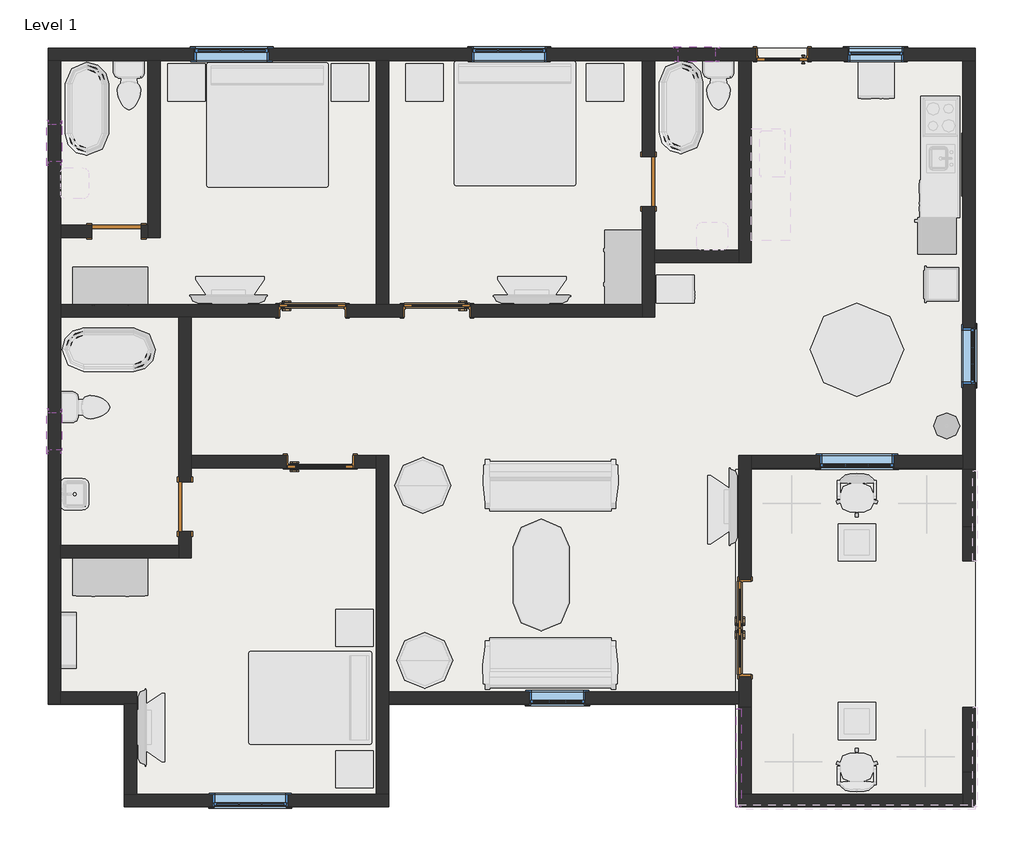
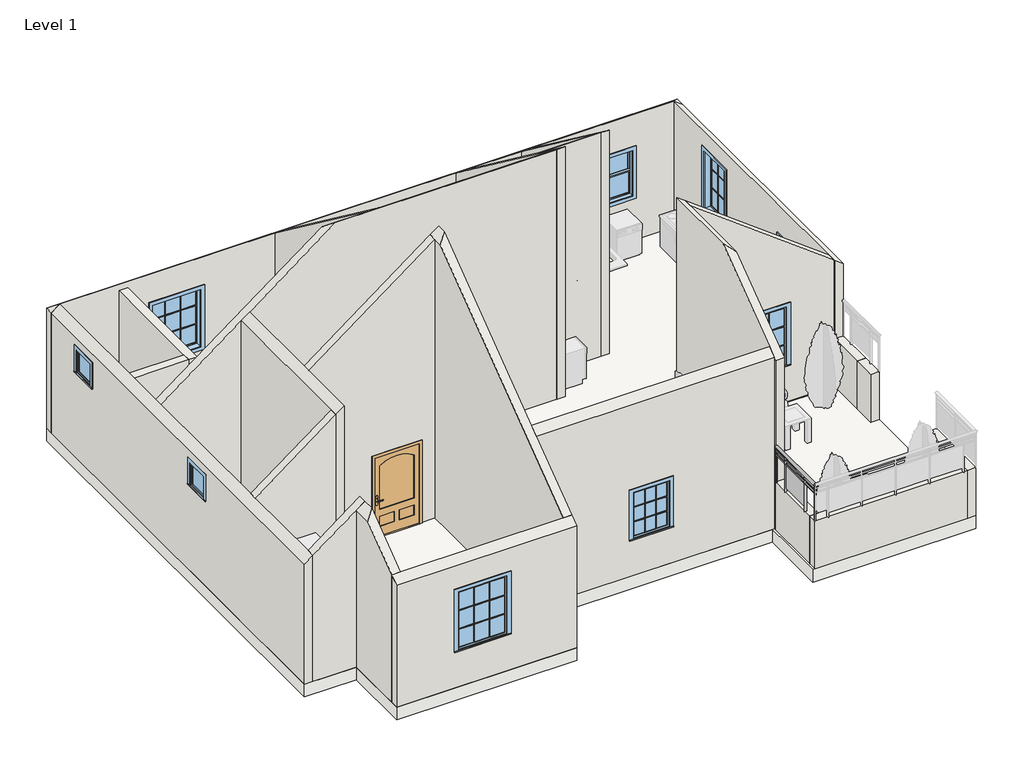
# One storey, part 1 of 2: 26 walls, 11 windows, 8 doors, 2 slabs, 1 railing.
"""IFC4 building model written with IfcOpenShell, lengths in millimetres."""

from ifc_helpers import new_model, si_unit, point, frame, origin, origin_with_axes, place, context, project, spatial, polyline, ellipse_curve, trimmed, outline, extrude, faceted_brep, transform, mapped, element, save
from ifc_brep_helpers import plane_surface, extruded_surface, advanced_brep
from components import door_fa6f8c62, door_3b8e8068, door_b03bd389, door_22967355, door_0d629d65, door_64d5ae29, window_29c06734, window_58e1470a, window_99fc0ff6, window_31198920, window_e41d21a6

model = new_model("IFC4")

# Units and contexts
model_context = context("Model", 3, world=origin())
ifc_project = project(units=[si_unit("LENGTHUNIT", "METRE", prefix="MILLI")], contexts=[model_context])

# Site, building, storey
site = spatial("IfcSite", under=ifc_project)
building = spatial("IfcBuilding", under=site)
storey = spatial("IfcBuildingStorey", under=building, Name="Level 1", Elevation=0.0)

# Doors
placement = place(None, origin())
door_shape = door_fa6f8c62(model_context)
element("IfcDoor", 1, ObjectType="42\" x 80\"", at=placement, inside=storey, context=model_context, shape_type="MappedRepresentation", body=[
    mapped(door_shape, transform((-8993.195199, 2667.0826725, 0.0), x_axis=(-1.0, 0.0, 0.0), y_axis=(0.0, -1.0, 0.0), z_axis=(0.0, 0.0, 1.0))),
])
door_2_shape = door_3b8e8068(model_context)
element("IfcDoor", 2, ObjectType="42\" x 80\"", at=placement, inside=storey, context=model_context, shape_type="MappedRepresentation", body=[
    mapped(door_2_shape, transform((-6961.195199, 2667.0826725, 0.0), x_axis=(1.0, 0.0, 0.0), y_axis=(0.0, 1.0, 0.0), z_axis=(0.0, 0.0, 1.0))),
])
element("IfcDoor", 3, ObjectType="42\" x 80\"", at=placement, inside=storey, context=model_context, shape_type="MappedRepresentation", body=[
    mapped(door_2_shape, transform((-8866.195199, 196.9326725, 0.0), x_axis=(-1.0, 0.0, 0.0), y_axis=(0.0, -1.0, 0.0), z_axis=(0.0, 0.0, 1.0))),
])
door_3_shape = door_b03bd389(model_context)
element("IfcDoor", 4, ObjectType="Door-Exterior-Double-Full Glass-Wood_Clad : 60\" x 80\"", at=placement, inside=storey, context=model_context, shape_type="MappedRepresentation", body=[
    mapped(door_3_shape, transform((-1935.170199, -2517.6923275, 0.0), x_axis=(0.0, 1.0, 0.0), y_axis=(-1.0, 0.0, 0.0), z_axis=(0.0, 0.0, 1.0))),
])
door_4_shape = door_22967355(model_context)
element("IfcDoor", 5, ObjectType="Door-Interior-Single-Full Glass-Wood : 32\" x 80\"", at=placement, inside=storey, context=model_context, shape_type="MappedRepresentation", body=[
    mapped(door_4_shape, transform((-1322.395199, 6851.7326725, 0.0), x_axis=(-1.0, 0.0, 0.0), y_axis=(0.0, -1.0, 0.0), z_axis=(0.0, 0.0, 1.0))),
])
door_5_shape = door_0d629d65(model_context)
element("IfcDoor", 6, ObjectType="Single-Flush : 32\" x 84\"", at=placement, inside=storey, context=model_context, shape_type="MappedRepresentation", body=[
    mapped(door_5_shape, transform((-11075.995199, -536.4923275, 0.0), x_axis=(0.0, -1.0, 0.0), y_axis=(1.0, 0.0, 0.0), z_axis=(0.0, 0.0, 1.0))),
])
door_6_shape = door_64d5ae29(model_context)
element("IfcDoor", 7, ObjectType="Single-Flush : 32\" x 84\"", at=placement, inside=storey, context=model_context, shape_type="MappedRepresentation", body=[
    mapped(door_6_shape, transform((-3506.795199, 4772.1076725, 0.0), x_axis=(0.0, -1.0, 0.0), y_axis=(1.0, 0.0, 0.0), z_axis=(0.0, 0.0, 1.0))),
])
element("IfcDoor", 8, ObjectType="Single-Flush : 32\" x 84\"", at=placement, inside=storey, context=model_context, shape_type="MappedRepresentation", body=[
    mapped(door_6_shape, transform((-12193.595199, 3959.3076725, 0.0), x_axis=(1.0, 0.0, 0.0), y_axis=(0.0, 1.0, 0.0), z_axis=(0.0, 0.0, 1.0))),
])

# Railing
element("IfcRailing", 9, ObjectType="Glass Panel - Bottom Fill", at=placement, inside=storey, context=model_context, shape_type="SolidModel", body=[
    advanced_brep(
    [(-1995.495199, -3838.4923275, 2133.6), (-2071.695199, -3838.4923275, 2133.6), (-1995.495199, -5438.6923275, 2133.6), (-2071.695199, -5438.6923275, 2133.6)],
    [
        (0, 1, ellipse_curve(frame((-2033.595199, -3838.4923275, 2133.6), z_axis=(0.0, 1.0, 0.0), x_axis=(-1.0, 0.0, 0.0)), 38.1, 28.575)),
        (1, 0, ellipse_curve(frame((-2033.595199, -3838.4923275, 2133.6), z_axis=(0.0, 1.0, 0.0), x_axis=(-1.0, 0.0, 0.0)), 38.1, 28.575)),
        (2, 3, ellipse_curve(frame((-2033.595199, -5438.6923275, 2133.6), z_axis=(0.0, -1.0, 0.0), x_axis=(-1.0, 0.0, 0.0)), 38.1, 28.575)),
        (3, 2, ellipse_curve(frame((-2033.595199, -5438.6923275, 2133.6), z_axis=(0.0, -1.0, 0.0), x_axis=(-1.0, 0.0, 0.0)), 38.1, 28.575)),
        (0, 2),
        (3, 1),
    ],
    [
        plane_surface(frame((-2033.595199, -3838.4923275, 2133.6), z_axis=(0.0, 1.0, 0.0), x_axis=(0.0, 0.0, -1.0))),
        plane_surface(frame((-2033.595199, -5438.6923275, 2133.6), z_axis=(0.0, -1.0, 0.0), x_axis=(0.0, 0.0, -1.0))),
        extruded_surface(trimmed(ellipse_curve(frame((-2033.595199, -5438.6923275, 2133.6), z_axis=(0.0, 1.0, 0.0), x_axis=(-1.0, 0.0, 0.0)), 38.1, 28.575), [point((-1995.495199, -5438.6923275, 2133.6))], [point((-2071.695199, -5438.6923275, 2133.6))], True, "CARTESIAN"), (0.0, 1600.1999999999998, 0.0), 1600.1999999999998),
        extruded_surface(trimmed(ellipse_curve(frame((-2033.595199, -5438.6923275, 2133.6), z_axis=(0.0, 1.0, 0.0), x_axis=(-1.0, 0.0, 0.0)), 38.1, 28.575), [point((-2071.695199, -5438.6923275, 2133.6))], [point((-1995.495199, -5438.6923275, 2133.6))], True, "CARTESIAN"), (0.0, 1600.1999999999998, 0.0), 1600.1999999999998),
    ],
    [
        (0, [[1, 2]]),
        (1, [[3, 4]]),
        (2, [[-1, 5, -4, 6]]),
        (3, [[-2, -6, -3, -5]]),
    ],
),
    extrude(outline(polyline([(-2046.295199, -3838.4923275), (-2020.895199, -3838.4923275), (-2020.895199, -5438.6923275), (-2046.295199, -5438.6923275), (-2046.295199, -3838.4923275)])), frame((0.0, 0.0, 2019.3), z_axis=(0.0, 0.0, 1.0), x_axis=(1.0, 0.0, 0.0)), (0.0, 0.0, 1.0), 25.4),
    extrude(outline(polyline([(-2046.295199, -3838.4923275), (-2020.895199, -3838.4923275), (-2020.895199, -5438.6923275), (-2046.295199, -5438.6923275), (-2046.295199, -3838.4923275)])), frame((0.0, 0.0, 1917.7), z_axis=(0.0, 0.0, 1.0), x_axis=(1.0, 0.0, 0.0)), (0.0, 0.0, 1.0), 25.4),
    extrude(outline(polyline([(-2058.995199, -5038.6423275), (-2008.195199, -5038.6423275), (-2008.195199, -5051.3423275), (-2058.995199, -5051.3423275), (-2058.995199, -5038.6423275)])), frame((0.0, 0.0, 1219.2), z_axis=(0.0, 0.0, 1.0), x_axis=(1.0, 0.0, 0.0)), (0.0, 0.0, 1.0), 885.6788223),
    extrude(outline(polyline([(-2027.060042, -4232.1923275), (-2027.060042, -5044.9923275), (-2033.410042, -5044.9923275), (-2033.410042, -4232.1923275), (-2027.060042, -4232.1923275)])), frame((0.0, 0.0, 1320.8), z_axis=(0.0, 0.0, 1.0), x_axis=(1.0, 0.0, 0.0)), (0.0, 0.0, 1.0), 596.9),
    extrude(outline(polyline([(-2058.995199, -4225.8423275), (-2008.195199, -4225.8423275), (-2008.195199, -4238.5423275), (-2058.995199, -4238.5423275), (-2058.995199, -4225.8423275)])), frame((0.0, 0.0, 1219.2), z_axis=(0.0, 0.0, 1.0), x_axis=(1.0, 0.0, 0.0)), (0.0, 0.0, 1.0), 885.6788223),
    extrude(outline(polyline([(-2043.120199, -5425.9923275), (-2024.070199, -5425.9923275), (-2024.070199, -5445.0423275), (-2043.120199, -5445.0423275), (-2043.120199, -5425.9923275)])), frame((0.0, 0.0, 1219.2), z_axis=(0.0, 0.0, 1.0), x_axis=(1.0, 0.0, 0.0)), (0.0, 0.0, 1.0), 885.6788223),
    extrude(outline(polyline([(-2043.120199, -3832.1423275), (-2024.070199, -3832.1423275), (-2024.070199, -3851.1923275), (-2043.120199, -3851.1923275), (-2043.120199, -3832.1423275)])), frame((0.0, 0.0, 1219.2), z_axis=(0.0, 0.0, 1.0), x_axis=(1.0, 0.0, 0.0)), (0.0, 0.0, 1.0), 885.6788223),
])

# Slabs
element("IfcSlab", 10, at=placement, inside=storey, context=model_context, shape_type="SweptSolid", body=[
    extrude(outline(polyline([(-13311.195199, -3762.2923275), (-13311.195199, 6956.5076725), (1827.204801, 6956.5076725), (1827.204801, 73.1076725), (-1855.795199, 73.1076725), (-1855.795199, -3762.2923275), (-7748.595199, -3762.2923275), (-7748.595199, -5438.6923275), (-12066.595199, -5438.6923275), (-12066.595199, -3762.2923275), (-13311.195199, -3762.2923275)])), frame((0.0, 0.0, -323.85), z_axis=(0.0, 0.0, 1.0), x_axis=(1.0, 0.0, 0.0)), (0.0, 0.0, 1.0), 323.85),
])
element("IfcSlab", 11, at=placement, inside=storey, context=model_context, shape_type="SweptSolid", body=[
    extrude(outline(polyline([(1827.204801, -5438.6923275), (-2084.395199, -5438.6923275), (-2084.395199, 73.1076725), (1827.204801, 73.1076725), (1827.204801, -5438.6923275)])), frame((0.0, 0.0, -323.85), z_axis=(0.0, 0.0, 1.0), x_axis=(1.0, 0.0, 0.0)), (0.0, 0.0, 1.0), 323.85),
])

# Walls
element("IfcWall", 12, ObjectType="Generic - 8\"", at=placement, inside=storey, context=model_context, shape_type="Brep", body=[
    faceted_brep([(1827.204801, 6753.3076725, 0.0), (1827.204801, 6753.3076725, 3048.0), (1624.004801, 6753.3076725, 3200.4), (-1830.395199, 6753.3076725, 3200.4), (-2033.595199, 6753.3076725, 3200.4), (-3405.195199, 6753.3076725, 3200.4), (-3608.395199, 6753.3076725, 3200.4), (-7748.595199, 6753.3076725, 3200.4), (-7951.795199, 6753.3076725, 3200.4), (-13107.995199, 6753.3076725, 3200.4), (-13311.195199, 6753.3076725, 3048.0), (-13311.195199, 6753.3076725, 0.0), (-13107.995199, 6753.3076725, 0.0), (-11685.595199, 6753.3076725, 0.0), (-11482.395199, 6753.3076725, 0.0), (-7951.795199, 6753.3076725, 0.0), (-7748.595199, 6753.3076725, 0.0), (-3608.395199, 6753.3076725, 0.0), (-3405.195199, 6753.3076725, 0.0), (-2033.595199, 6753.3076725, 0.0), (-1830.395199, 6753.3076725, 0.0), (-1754.195199, 6753.3076725, 0.0), (-1754.195199, 6753.3076725, 2057.4), (-890.595199, 6753.3076725, 2057.4), (-890.595199, 6753.3076725, 0.0), (1624.004801, 6753.3076725, 0.0), (-9704.395199, 6753.3076725, 2438.4), (-9704.395199, 6753.3076725, 914.4), (-10923.595199, 6753.3076725, 914.4), (-10923.595199, 6753.3076725, 2438.4), (-5170.495199, 6753.3076725, 2438.4), (-5170.495199, 6753.3076725, 914.4), (-6389.695199, 6753.3076725, 914.4), (-6389.695199, 6753.3076725, 2438.4), (658.804801, 6753.3076725, 2336.8), (658.804801, 6753.3076725, 1117.6), (-255.595199, 6753.3076725, 1117.6), (-255.595199, 6753.3076725, 2336.8), (-2414.595199, 6753.3076725, 2768.6), (-2414.595199, 6753.3076725, 2159.0), (-3024.195199, 6753.3076725, 2159.0), (-3024.195199, 6753.3076725, 2768.6), (-13311.195199, 6956.5076725, 3048.0), (1827.204801, 6956.5076725, 3048.0), (1827.204801, 6956.5076725, 0.0), (-890.595199, 6956.5076725, 0.0), (-890.595199, 6956.5076725, 2057.4), (-1754.195199, 6956.5076725, 2057.4), (-1754.195199, 6956.5076725, 0.0), (-13311.195199, 6956.5076725, 0.0), (-9704.395199, 6956.5076725, 2438.4), (-10923.595199, 6956.5076725, 2438.4), (-10923.595199, 6956.5076725, 914.4), (-9704.395199, 6956.5076725, 914.4), (-5170.495199, 6956.5076725, 2438.4), (-6389.695199, 6956.5076725, 2438.4), (-6389.695199, 6956.5076725, 914.4), (-5170.495199, 6956.5076725, 914.4), (658.804801, 6956.5076725, 2336.8), (-255.595199, 6956.5076725, 2336.8), (-255.595199, 6956.5076725, 1117.6), (658.804801, 6956.5076725, 1117.6), (-2414.595199, 6956.5076725, 2768.6), (-3024.195199, 6956.5076725, 2768.6), (-3024.195199, 6956.5076725, 2159.0), (-2414.595199, 6956.5076725, 2159.0)], [[[0, 1, 2, 3, 4, 5, 6, 7, 8, 9, 10, 11, 12, 13, 14, 15, 16, 17, 18, 19, 20, 21, 22, 23, 24, 25], [26, 27, 28, 29], [30, 31, 32, 33], [34, 35, 36, 37], [38, 39, 40, 41]], [[42, 43, 44, 45, 46, 47, 48, 49], [50, 51, 52, 53], [54, 55, 56, 57], [58, 59, 60, 61], [62, 63, 64, 65]], [[44, 0, 25, 24, 45]], [[11, 49, 48, 21, 20, 19, 18, 17, 16, 15, 14, 13, 12]], [[1, 0, 44, 43]], [[11, 10, 42, 49]], [[42, 10, 9]], [[43, 42, 9, 8, 7, 6, 5, 4, 3, 2]], [[1, 43, 2]], [[47, 22, 21, 48]], [[22, 47, 46, 23]], [[23, 46, 45, 24]], [[27, 26, 50, 53]], [[28, 27, 53, 52]], [[29, 28, 52, 51]], [[26, 29, 51, 50]], [[31, 30, 54, 57]], [[32, 31, 57, 56]], [[33, 32, 56, 55]], [[30, 33, 55, 54]], [[35, 34, 58, 61]], [[36, 35, 61, 60]], [[37, 36, 60, 59]], [[34, 37, 59, 58]], [[39, 38, 62, 65]], [[40, 39, 65, 64]], [[41, 40, 64, 63]], [[38, 41, 63, 62]]]),
])
element("IfcWall", 13, ObjectType="Generic - 8\"", at=placement, inside=storey, context=model_context, shape_type="Brep", body=[
    faceted_brep([(1624.004801, 6753.3076725, 0.0), (1624.004801, 301.7076725, 0.0), (1624.004801, 98.5076725, 0.0), (1624.004801, 73.1076725, 0.0), (1624.004801, 73.1076725, 1219.2), (1624.004801, 73.1076725, 3200.4), (1624.004801, 98.5076725, 3200.4), (1624.004801, 301.7076725, 3200.4), (1624.004801, 6753.3076725, 3200.4), (1624.004801, 4594.3076725, 2743.2), (1624.004801, 4594.3076725, 1219.2), (1624.004801, 5508.7076725, 1219.2), (1624.004801, 5508.7076725, 2743.2), (1624.004801, 1470.1076725, 2438.4), (1624.004801, 1470.1076725, 914.4), (1624.004801, 2384.5076725, 914.4), (1624.004801, 2384.5076725, 2438.4), (1827.204801, 6753.3076725, 0.0), (1827.204801, 6753.3076725, 3048.0), (1827.204801, 73.1076725, 3048.0), (1827.204801, 73.1076725, 1219.2), (1827.204801, 73.1076725, 0.0), (1827.204801, 4594.3076725, 2743.2), (1827.204801, 5508.7076725, 2743.2), (1827.204801, 5508.7076725, 1219.2), (1827.204801, 4594.3076725, 1219.2), (1827.204801, 1470.1076725, 2438.4), (1827.204801, 2384.5076725, 2438.4), (1827.204801, 2384.5076725, 914.4), (1827.204801, 1470.1076725, 914.4)], [[[0, 1, 2, 3, 4, 5, 6, 7, 8], [9, 10, 11, 12], [13, 14, 15, 16]], [[17, 18, 19, 20, 21], [22, 23, 24, 25], [26, 27, 28, 29]], [[3, 2, 1, 0, 17, 21]], [[5, 4, 3, 21, 20, 19]], [[0, 8, 18, 17]], [[8, 7, 6, 5, 19, 18]], [[10, 9, 22, 25]], [[11, 10, 25, 24]], [[12, 11, 24, 23]], [[9, 12, 23, 22]], [[14, 13, 26, 29]], [[15, 14, 29, 28]], [[16, 15, 28, 27]], [[13, 16, 27, 26]]]),
])
element("IfcWall", 14, ObjectType="Generic - 8\"", at=placement, inside=storey, context=model_context, shape_type="Brep", body=[
    faceted_brep([(1624.004801, -5235.4923275, 0.0), (-1830.395199, -5235.4923275, 0.0), (-2033.595199, -5235.4923275, 0.0), (-2033.595199, -5235.4923275, 1219.2), (-1830.395199, -5235.4923275, 1219.2), (1624.004801, -5235.4923275, 1219.2), (1624.004801, -5438.6923275, 0.0), (1624.004801, -5438.6923275, 1219.2), (-2033.595199, -5438.6923275, 1219.2), (-2033.595199, -5438.6923275, 0.0)], [[[0, 1, 2, 3, 4, 5]], [[6, 7, 8, 9]], [[2, 1, 0, 6, 9]], [[5, 4, 3, 8, 7]], [[0, 5, 7, 6]], [[3, 2, 9, 8]]]),
])
element("IfcWall", 15, ObjectType="Generic - 8\"", at=placement, inside=storey, context=model_context, shape_type="Brep", body=[
    faceted_brep([(-13107.995199, -3762.2923275, 0.0), (-12066.595199, -3762.2923275, 0.0), (-11863.395199, -3762.2923275, 0.0), (-11863.395199, -3762.2923275, 4133.85), (-12066.595199, -3762.2923275, 3981.45), (-13107.995199, -3762.2923275, 3200.4), (-13107.995199, -3559.0923275, 0.0), (-13107.995199, -3559.0923275, 3200.4), (-11863.395199, -3559.0923275, 4133.85), (-11863.395199, -3559.0923275, 0.0)], [[[0, 1, 2, 3, 4, 5]], [[6, 7, 8, 9]], [[2, 1, 0, 6, 9]], [[3, 2, 9, 8]], [[0, 5, 7, 6]], [[5, 4, 3, 8, 7]]]),
])
element("IfcWall", 16, ObjectType="Generic - 8\"", at=placement, inside=storey, context=model_context, shape_type="Brep", body=[
    faceted_brep([(-12066.595199, -3762.2923275, 0.0), (-12066.595199, -5235.4923275, 0.0), (-12066.595199, -5235.4923275, 3238.5), (-12066.595199, -4244.8923275, 3981.45), (-12066.595199, -3762.2923275, 3981.45), (-11863.395199, -3762.2923275, 0.0), (-11863.395199, -3762.2923275, 4133.85), (-11863.395199, -4041.6923275, 4133.85), (-11863.395199, -5235.4923275, 3238.5), (-11863.395199, -5235.4923275, 0.0)], [[[0, 1, 2, 3, 4]], [[5, 6, 7, 8, 9]], [[1, 0, 5, 9]], [[0, 4, 6, 5]], [[2, 1, 9, 8]], [[4, 3, 7, 6]], [[3, 2, 8, 7]]]),
])
element("IfcWall", 17, ObjectType="Generic - 8\"", at=placement, inside=storey, context=model_context, shape_type="Brep", body=[
    faceted_brep([(-13107.995199, -3762.2923275, 0.0), (-13107.995199, -3559.0923275, 0.0), (-13107.995199, -1374.6923275, 0.0), (-13107.995199, -1171.4923275, 0.0), (-13107.995199, 2562.3076725, 0.0), (-13107.995199, 2765.5076725, 0.0), (-13107.995199, 3857.7076725, 0.0), (-13107.995199, 4060.9076725, 0.0), (-13107.995199, 6753.3076725, 0.0), (-13107.995199, 6753.3076725, 3200.4), (-13107.995199, 2765.5076725, 3200.4), (-13107.995199, 2562.3076725, 3200.4), (-13107.995199, -1171.4923275, 3200.4), (-13107.995199, -1374.6923275, 3200.4), (-13107.995199, -3559.0923275, 3200.4), (-13107.995199, -3762.2923275, 3200.4), (-13107.995199, 1000.2076725, 2768.6), (-13107.995199, 1000.2076725, 2159.0), (-13107.995199, 390.6076725, 2159.0), (-13107.995199, 390.6076725, 2768.6), (-13107.995199, 5711.9076725, 2768.6), (-13107.995199, 5711.9076725, 2159.0), (-13107.995199, 5102.3076725, 2159.0), (-13107.995199, 5102.3076725, 2768.6), (-13311.195199, -3762.2923275, 0.0), (-13311.195199, -3762.2923275, 3048.0), (-13311.195199, 6753.3076725, 3048.0), (-13311.195199, 6753.3076725, 0.0), (-13311.195199, 1000.2076725, 2768.6), (-13311.195199, 390.6076725, 2768.6), (-13311.195199, 390.6076725, 2159.0), (-13311.195199, 1000.2076725, 2159.0), (-13311.195199, 5711.9076725, 2768.6), (-13311.195199, 5102.3076725, 2768.6), (-13311.195199, 5102.3076725, 2159.0), (-13311.195199, 5711.9076725, 2159.0)], [[[0, 1, 2, 3, 4, 5, 6, 7, 8, 9, 10, 11, 12, 13, 14, 15], [16, 17, 18, 19], [20, 21, 22, 23]], [[24, 25, 26, 27], [28, 29, 30, 31], [32, 33, 34, 35]], [[8, 7, 6, 5, 4, 3, 2, 1, 0, 24, 27]], [[9, 8, 27, 26]], [[0, 15, 25, 24]], [[15, 14, 13, 12, 11, 10, 9, 26, 25]], [[17, 16, 28, 31]], [[18, 17, 31, 30]], [[19, 18, 30, 29]], [[16, 19, 29, 28]], [[21, 20, 32, 35]], [[22, 21, 35, 34]], [[23, 22, 34, 33]], [[20, 23, 33, 32]]]),
])
element("IfcWall", 18, ObjectType="Generic - 8\"", at=placement, inside=storey, context=model_context, shape_type="Brep", body=[
    faceted_brep([(-7951.795199, 6753.3076725, 0.0), (-7951.795199, 2765.5076725, 0.0), (-7951.795199, 2765.5076725, 6191.25), (-7951.795199, 6753.3076725, 3200.4), (-7748.595199, 6753.3076725, 0.0), (-7748.595199, 6753.3076725, 3200.4), (-7748.595199, 2765.5076725, 6191.25), (-7748.595199, 2765.5076725, 0.0), (-7875.595199, 2765.5076725, 0.0)], [[[0, 1, 2, 3]], [[4, 5, 6, 7]], [[1, 0, 4, 7, 8]], [[0, 3, 5, 4]], [[2, 1, 8, 7, 6]], [[3, 2, 6, 5]]]),
])
element("IfcWall", 19, ObjectType="Generic - 8\"", at=placement, inside=storey, context=model_context, shape_type="Brep", body=[
    faceted_brep([(-7748.595199, -3762.2923275, 0.0), (-2033.595199, -3762.2923275, 0.0), (-2033.595199, -3762.2923275, 4343.4), (-7748.595199, -3762.2923275, 4343.4), (-5449.895199, -3762.2923275, 2133.6), (-4535.495199, -3762.2923275, 2133.6), (-4535.495199, -3762.2923275, 914.4), (-5449.895199, -3762.2923275, 914.4), (-7748.595199, -3559.0923275, 0.0), (-7748.595199, -3559.0923275, 4495.8), (-2033.595199, -3559.0923275, 4495.8), (-2033.595199, -3559.0923275, 0.0), (-5449.895199, -3559.0923275, 2133.6), (-5449.895199, -3559.0923275, 914.4), (-4535.495199, -3559.0923275, 914.4), (-4535.495199, -3559.0923275, 2133.6)], [[[0, 1, 2, 3], [4, 5, 6, 7]], [[8, 9, 10, 11], [12, 13, 14, 15]], [[1, 0, 8, 11]], [[0, 3, 9, 8]], [[2, 1, 11, 10]], [[3, 2, 10, 9]], [[13, 12, 4, 7]], [[14, 13, 7, 6]], [[15, 14, 6, 5]], [[12, 15, 5, 4]]]),
])
element("IfcWall", 20, ObjectType="Generic - 8\"", at=placement, inside=storey, context=model_context, shape_type="SweptSolid", body=[
    extrude(outline(polyline([(-1830.395199, -3813.0923275), (-1830.395199, -5235.4923275), (-2033.595199, -5235.4923275), (-2033.595199, -3813.0923275), (-1830.395199, -3813.0923275)])), origin_with_axes(), (0.0, 0.0, 1.0), 1219.2),
])
element("IfcWall", 21, ObjectType="Generic - 8\"", at=placement, inside=storey, context=model_context, shape_type="SweptSolid", body=[
    extrude(outline(polyline([(0.0, -1830.395199), (0.0, 1624.004801), (3200.4, 1624.004801), (5791.2, -1830.395199), (0.0, -1830.395199)]), holes=[polyline([(2438.4, -712.795199), (2438.4, 506.404801), (914.4, 506.404801), (914.4, -712.795199), (2438.4, -712.795199)])]), frame((0.0, 98.5076725, 0.0), z_axis=(0.0, 1.0, 0.0), x_axis=(0.0, 0.0, 1.0)), (0.0, 0.0, 1.0), 203.2),
])
element("IfcWall", 22, ObjectType="Generic - 8\"", at=placement, inside=storey, context=model_context, shape_type="Brep", body=[
    faceted_brep([(-13107.995199, 2562.3076725, 3200.4), (-13107.995199, 2562.3076725, 0.0), (-11177.595199, 2562.3076725, 0.0), (-10974.395199, 2562.3076725, 0.0), (-9551.995199, 2562.3076725, 0.0), (-9551.995199, 2562.3076725, 2057.4), (-8434.395199, 2562.3076725, 2057.4), (-8434.395199, 2562.3076725, 0.0), (-7519.995199, 2562.3076725, 0.0), (-7519.995199, 2562.3076725, 2057.4), (-6402.395199, 2562.3076725, 2057.4), (-6402.395199, 2562.3076725, 0.0), (-3608.395199, 2562.3076725, 0.0), (-3608.395199, 2562.3076725, 6343.65), (-8916.995199, 2562.3076725, 6343.65), (-10974.395199, 2562.3076725, 4800.6), (-11177.595199, 2562.3076725, 4648.2), (-13107.995199, 2765.5076725, 0.0), (-13107.995199, 2765.5076725, 3200.4), (-9120.195199, 2765.5076725, 6191.25), (-7951.795199, 2765.5076725, 6191.25), (-7748.595199, 2765.5076725, 6191.25), (-3608.395199, 2765.5076725, 6191.25), (-3608.395199, 2765.5076725, 0.0), (-6402.395199, 2765.5076725, 0.0), (-6402.395199, 2765.5076725, 2057.4), (-7519.995199, 2765.5076725, 2057.4), (-7519.995199, 2765.5076725, 0.0), (-7748.595199, 2765.5076725, 0.0), (-7951.795199, 2765.5076725, 0.0), (-8434.395199, 2765.5076725, 0.0), (-8434.395199, 2765.5076725, 2057.4), (-9551.995199, 2765.5076725, 2057.4), (-9551.995199, 2765.5076725, 0.0)], [[[0, 1, 2, 3, 4, 5, 6, 7, 8, 9, 10, 11, 12, 13, 14, 15, 16]], [[17, 18, 19, 20, 21, 22, 23, 24, 25, 26, 27, 28, 29, 30, 31, 32, 33]], [[1, 17, 33, 4, 3, 2]], [[23, 12, 11, 24]], [[7, 30, 29, 28, 27, 8]], [[1, 0, 18, 17]], [[13, 12, 23, 22]], [[18, 0, 16, 15, 14, 19]], [[13, 22, 21, 20, 19, 14]], [[32, 5, 4, 33]], [[5, 32, 31, 6]], [[6, 31, 30, 7]], [[10, 25, 24, 11]], [[25, 10, 9, 26]], [[26, 9, 8, 27]]]),
])
element("IfcWall", 23, ObjectType="Generic - 8\"", at=placement, inside=storey, context=model_context, shape_type="Brep", body=[
    faceted_brep([(-11177.595199, -942.8923275, 2133.6), (-11177.595199, -942.8923275, 0.0), (-11177.595199, -1171.4923275, 0.0), (-11177.595199, -1374.6923275, 0.0), (-11177.595199, -1374.6923275, 4648.2), (-11177.595199, -1171.4923275, 4648.2), (-11177.595199, 2562.3076725, 4648.2), (-11177.595199, 2562.3076725, 0.0), (-11177.595199, -130.0923275, 0.0), (-11177.595199, -130.0923275, 2133.6), (-10974.395199, -1374.6923275, 0.0), (-10974.395199, -942.8923275, 0.0), (-10974.395199, -942.8923275, 2133.6), (-10974.395199, -130.0923275, 2133.6), (-10974.395199, -130.0923275, 0.0), (-10974.395199, 98.5076725, 0.0), (-10974.395199, 301.7076725, 0.0), (-10974.395199, 2562.3076725, 0.0), (-10974.395199, 2562.3076725, 4800.6), (-10974.395199, 301.7076725, 4800.6), (-10974.395199, 98.5076725, 4800.6), (-10974.395199, -1374.6923275, 4800.6)], [[[0, 1, 2, 3, 4, 5, 6, 7, 8, 9]], [[10, 11, 12, 13, 14, 15, 16, 17, 18, 19, 20, 21]], [[8, 7, 17, 16, 15, 14]], [[3, 2, 1, 11, 10]], [[7, 6, 18, 17]], [[4, 3, 10, 21]], [[6, 5, 4, 21, 20, 19, 18]], [[12, 11, 1, 0]], [[13, 12, 0, 9]], [[14, 13, 9, 8]]]),
])
element("IfcWall", 24, ObjectType="Generic - 8\"", at=placement, inside=storey, context=model_context, shape_type="SweptSolid", body=[
    extrude(outline(polyline([(0.0, -11177.595199), (4648.2, -11177.595199), (3200.4, -13107.995199), (0.0, -13107.995199), (0.0, -11177.595199)])), frame((0.0, -1374.6923275, 0.0), z_axis=(0.0, 1.0, 0.0), x_axis=(0.0, 0.0, 1.0)), (0.0, 0.0, 1.0), 203.2),
])
element("IfcWall", 25, ObjectType="Generic - 8\"", at=placement, inside=storey, context=model_context, shape_type="SweptSolid", body=[
    extrude(outline(polyline([(4800.6, -10974.395199), (0.0, -10974.395199), (0.0, -9424.995199), (2057.4, -9424.995199), (2057.4, -8307.395199), (0.0, -8307.395199), (0.0, -7951.795199), (7067.55, -7951.795199), (4800.6, -10974.395199)])), frame((0.0, 98.5076725, 0.0), z_axis=(0.0, 1.0, 0.0), x_axis=(0.0, 0.0, 1.0)), (0.0, 0.0, 1.0), 203.2),
])
element("IfcWall", 26, ObjectType="Generic - 8\"", at=placement, inside=storey, context=model_context, shape_type="Brep", body=[
    faceted_brep([(-7951.795199, 301.7076725, 0.0), (-7951.795199, 98.5076725, 0.0), (-7951.795199, -5235.4923275, 0.0), (-7951.795199, -5235.4923275, 3238.5), (-7951.795199, -130.0923275, 7067.55), (-7951.795199, 98.5076725, 7067.55), (-7951.795199, 301.7076725, 7067.55), (-7748.595199, 301.7076725, 0.0), (-7748.595199, 301.7076725, 7219.95), (-7748.595199, 73.1076725, 7219.95), (-7748.595199, -3559.0923275, 4495.8), (-7748.595199, -3762.2923275, 4343.4), (-7748.595199, -5235.4923275, 3238.5), (-7748.595199, -5235.4923275, 0.0), (-7748.595199, -3762.2923275, 0.0), (-7748.595199, -3559.0923275, 0.0)], [[[0, 1, 2, 3, 4, 5, 6]], [[7, 8, 9, 10, 11, 12, 13, 14, 15]], [[2, 1, 0, 7, 15, 14, 13]], [[0, 6, 8, 7]], [[3, 2, 13, 12]], [[6, 5, 4, 9, 8]], [[4, 3, 12, 11, 10, 9]]]),
])
element("IfcWall", 27, ObjectType="Generic - 8\"", at=placement, inside=storey, context=model_context, shape_type="Brep", body=[
    faceted_brep([(-3608.395199, 4365.7076725, 2133.6), (-3608.395199, 4365.7076725, 0.0), (-3608.395199, 2765.5076725, 0.0), (-3608.395199, 2562.3076725, 0.0), (-3608.395199, 2562.3076725, 6343.65), (-3608.395199, 2765.5076725, 6191.25), (-3608.395199, 6753.3076725, 3200.4), (-3608.395199, 6753.3076725, 0.0), (-3608.395199, 5178.5076725, 0.0), (-3608.395199, 5178.5076725, 2133.6), (-3405.195199, 2562.3076725, 0.0), (-3405.195199, 3451.3076725, 0.0), (-3405.195199, 3654.5076725, 0.0), (-3405.195199, 4365.7076725, 0.0), (-3405.195199, 4365.7076725, 2133.6), (-3405.195199, 5178.5076725, 2133.6), (-3405.195199, 5178.5076725, 0.0), (-3405.195199, 6753.3076725, 0.0), (-3405.195199, 6753.3076725, 3200.4), (-3405.195199, 3654.5076725, 5524.5), (-3405.195199, 3451.3076725, 5676.9), (-3405.195199, 2562.3076725, 6343.65)], [[[0, 1, 2, 3, 4, 5, 6, 7, 8, 9]], [[10, 11, 12, 13, 14, 15, 16, 17, 18, 19, 20, 21]], [[8, 7, 17, 16]], [[3, 2, 1, 13, 12, 11, 10]], [[7, 6, 18, 17]], [[4, 3, 10, 21]], [[6, 5, 4, 21, 20, 19, 18]], [[14, 13, 1, 0]], [[15, 14, 0, 9]], [[16, 15, 9, 8]]]),
])
element("IfcWall", 28, ObjectType="Generic - 8\"", at=placement, inside=storey, context=model_context, shape_type="Brep", body=[
    faceted_brep([(-2033.595199, 6753.3076725, 0.0), (-2033.595199, 3654.5076725, 0.0), (-2033.595199, 3451.3076725, 0.0), (-2033.595199, 3451.3076725, 5676.9), (-2033.595199, 3654.5076725, 5524.5), (-2033.595199, 6753.3076725, 3200.4), (-1830.395199, 6753.3076725, 0.0), (-1830.395199, 6753.3076725, 3200.4), (-1830.395199, 3451.3076725, 5676.9), (-1830.395199, 3451.3076725, 0.0)], [[[0, 1, 2, 3, 4, 5]], [[6, 7, 8, 9]], [[2, 1, 0, 6, 9]], [[0, 5, 7, 6]], [[3, 2, 9, 8]], [[5, 4, 3, 8, 7]]]),
])
element("IfcWall", 29, ObjectType="Generic - 8\"", at=placement, inside=storey, context=model_context, shape_type="SweptSolid", body=[
    extrude(outline(polyline([(3654.5076725, 5524.5), (3654.5076725, 0.0), (3451.3076725, 0.0), (3451.3076725, 5676.9), (3654.5076725, 5524.5)])), frame((-3405.195199, 0.0, 0.0), z_axis=(1.0, 0.0, 0.0), x_axis=(0.0, 1.0, 0.0)), (0.0, 0.0, 1.0), 1371.6),
])
element("IfcWall", 30, ObjectType="Generic - 8\"", at=placement, inside=storey, context=model_context, shape_type="Brep", body=[
    faceted_brep([(-7748.595199, -5235.4923275, 0.0), (-7951.795199, -5235.4923275, 0.0), (-11863.395199, -5235.4923275, 0.0), (-12066.595199, -5235.4923275, 0.0), (-12066.595199, -5235.4923275, 3238.5), (-11863.395199, -5235.4923275, 3238.5), (-7951.795199, -5235.4923275, 3238.5), (-7748.595199, -5235.4923275, 3238.5), (-10618.795199, -5235.4923275, 2438.4), (-10618.795199, -5235.4923275, 914.4), (-9399.595199, -5235.4923275, 914.4), (-9399.595199, -5235.4923275, 2438.4), (-7748.595199, -5438.6923275, 0.0), (-7748.595199, -5438.6923275, 3086.1), (-12066.595199, -5438.6923275, 3086.1), (-12066.595199, -5438.6923275, 0.0), (-10618.795199, -5438.6923275, 2438.4), (-9399.595199, -5438.6923275, 2438.4), (-9399.595199, -5438.6923275, 914.4), (-10618.795199, -5438.6923275, 914.4)], [[[0, 1, 2, 3, 4, 5, 6, 7], [8, 9, 10, 11]], [[12, 13, 14, 15], [16, 17, 18, 19]], [[3, 2, 1, 0, 12, 15]], [[0, 7, 13, 12]], [[4, 3, 15, 14]], [[7, 6, 5, 4, 14, 13]], [[9, 8, 16, 19]], [[10, 9, 19, 18]], [[11, 10, 18, 17]], [[8, 11, 17, 16]]]),
])
element("IfcWall", 31, ObjectType="Generic - 8\"", at=placement, inside=storey, context=model_context, shape_type="SweptSolid", body=[
    extrude(outline(polyline([(1624.004801, -866.6923275), (1624.004801, 73.1076725), (1827.204801, 73.1076725), (1827.204801, -866.6923275), (1624.004801, -866.6923275)])), origin_with_axes(), (0.0, 0.0, 1.0), 1219.2),
])
element("IfcWall", 32, ObjectType="Generic - 8\"", at=placement, inside=storey, context=model_context, shape_type="Brep", body=[
    faceted_brep([(-1830.395199, -3813.0923275, 4305.3), (-1830.395199, -3813.0923275, 1219.2), (-1830.395199, -3813.0923275, 0.0), (-1830.395199, -3305.0923275, 0.0), (-1830.395199, -3305.0923275, 2057.4), (-1830.395199, -1730.2923275, 2057.4), (-1830.395199, -1730.2923275, 0.0), (-1830.395199, 98.5076725, 0.0), (-1830.395199, 301.7076725, 0.0), (-1830.395199, 301.7076725, 5791.2), (-1830.395199, 98.5076725, 5791.2), (-1830.395199, -1831.8923275, 5791.2), (-2033.595199, -3813.0923275, 0.0), (-2033.595199, -3813.0923275, 1219.2), (-2033.595199, -3813.0923275, 4305.3), (-2033.595199, -3762.2923275, 4343.4), (-2033.595199, -3559.0923275, 4495.8), (-2033.595199, -1628.6923275, 5943.6), (-2033.595199, 301.7076725, 5943.6), (-2033.595199, 301.7076725, 0.0), (-2033.595199, -1730.2923275, 0.0), (-2033.595199, -1730.2923275, 2057.4), (-2033.595199, -3305.0923275, 2057.4), (-2033.595199, -3305.0923275, 0.0), (-2033.595199, -3559.0923275, 0.0), (-2033.595199, -3762.2923275, 0.0)], [[[0, 1, 2, 3, 4, 5, 6, 7, 8, 9, 10, 11]], [[12, 13, 14, 15, 16, 17, 18, 19, 20, 21, 22, 23, 24, 25]], [[19, 8, 7, 6, 20]], [[2, 12, 25, 24, 23, 3]], [[2, 1, 0, 14, 13, 12]], [[9, 8, 19, 18]], [[14, 0, 11, 17, 16, 15]], [[9, 18, 17, 11, 10]], [[5, 21, 20, 6]], [[21, 5, 4, 22]], [[22, 4, 3, 23]]]),
])
element("IfcWall", 33, ObjectType="Generic - 8\"", at=placement, inside=storey, context=model_context, shape_type="Brep", body=[
    faceted_brep([(1624.004801, -4879.8923275, 0.0), (1624.004801, -5235.4923275, 0.0), (1624.004801, -5438.6923275, 0.0), (1624.004801, -5438.6923275, 1219.2), (1624.004801, -5235.4923275, 1219.2), (1624.004801, -4879.8923275, 1219.2), (1827.204801, -4879.8923275, 0.0), (1827.204801, -4879.8923275, 1219.2), (1827.204801, -5438.6923275, 1219.2), (1827.204801, -5438.6923275, 0.0)], [[[0, 1, 2, 3, 4, 5]], [[6, 7, 8, 9]], [[2, 1, 0, 6, 9]], [[5, 4, 3, 8, 7]], [[0, 5, 7, 6]], [[3, 2, 9, 8]]]),
])
element("IfcWall", 34, ObjectType="Generic - 8\"", at=placement, inside=storey, context=model_context, shape_type="SweptSolid", body=[
    extrude(outline(polyline([(1827.204801, -3813.0923275), (1827.204801, -4879.8923275), (1624.004801, -4879.8923275), (1624.004801, -3813.0923275), (1827.204801, -3813.0923275)])), origin_with_axes(), (0.0, 0.0, 1.0), 1219.2),
])
element("IfcWall", 35, ObjectType="Generic - 8\"", at=placement, inside=storey, context=model_context, shape_type="SweptSolid", body=[
    extrude(outline(polyline([(1624.004801, -1425.4923275), (1624.004801, -866.6923275), (1827.204801, -866.6923275), (1827.204801, -1425.4923275), (1624.004801, -1425.4923275)])), origin_with_axes(), (0.0, 0.0, 1.0), 1219.2),
])
element("IfcWall", 36, ObjectType="Generic - 8\"", at=placement, inside=storey, context=model_context, shape_type="Brep", body=[
    faceted_brep([(-11685.595199, 6753.3076725, 0.0), (-11685.595199, 4060.9076725, 0.0), (-11685.595199, 3857.7076725, 0.0), (-11685.595199, 3857.7076725, 3048.0), (-11685.595199, 4060.9076725, 3048.0), (-11685.595199, 6753.3076725, 3048.0), (-11482.395199, 6753.3076725, 0.0), (-11482.395199, 6753.3076725, 3048.0), (-11482.395199, 3857.7076725, 3048.0), (-11482.395199, 3857.7076725, 0.0)], [[[0, 1, 2, 3, 4, 5]], [[6, 7, 8, 9]], [[2, 1, 0, 6, 9]], [[5, 4, 3, 8, 7]], [[0, 5, 7, 6]], [[3, 2, 9, 8]]]),
])
element("IfcWall", 37, ObjectType="Generic - 8\"", at=placement, inside=storey, context=model_context, shape_type="SweptSolid", body=[
    extrude(outline(polyline([(2133.6, -11787.195199), (0.0, -11787.195199), (0.0, -11685.595199), (3048.0, -11685.595199), (3048.0, -13107.995199), (0.0, -13107.995199), (0.0, -12599.995199), (2133.6, -12599.995199), (2133.6, -11787.195199)])), frame((0.0, 3857.7076725, 0.0), z_axis=(0.0, 1.0, 0.0), x_axis=(0.0, 0.0, 1.0)), (0.0, 0.0, 1.0), 203.2),
])

# Windows
window_shape = window_29c06734(model_context)
element("IfcWindow", 38, ObjectType="Casement 3x3 with Trim : 36\" x 48\"", at=placement, inside=storey, context=model_context, shape_type="MappedRepresentation", body=[
    mapped(window_shape, transform((-4992.695199, -3660.6923275, 0.0), x_axis=(-1.0, 0.0, 0.0), y_axis=(0.0, -1.0, 0.0), z_axis=(0.0, 0.0, 1.0))),
])
window_2_shape = window_58e1470a(model_context)
element("IfcWindow", 39, ObjectType="Casement 3x3 with Trim : 36\" x 60\"", at=placement, inside=storey, context=model_context, shape_type="MappedRepresentation", body=[
    mapped(window_2_shape, transform((1725.604801, 5051.5076725, 609.6), x_axis=(0.0, -1.0, 0.0), y_axis=(1.0, 0.0, 0.0), z_axis=(0.0, 0.0, 1.0))),
])
element("IfcWindow", 40, ObjectType="Casement 3x3 with Trim : 36\" x 60\"", at=placement, inside=storey, context=model_context, shape_type="MappedRepresentation", body=[
    mapped(window_2_shape, transform((1725.604801, 1927.3076725, 304.8), x_axis=(0.0, -1.0, 0.0), y_axis=(1.0, 0.0, 0.0), z_axis=(0.0, 0.0, 1.0))),
])
window_3_shape = window_99fc0ff6(model_context)
element("IfcWindow", 41, ObjectType="Casement 3x3 with Trim : 48\" x 60\"", at=placement, inside=storey, context=model_context, shape_type="MappedRepresentation", body=[
    mapped(window_3_shape, transform((-10009.195199, -5337.0923275, 609.6), x_axis=(-1.0, 0.0, 0.0), y_axis=(0.0, -1.0, 0.0), z_axis=(0.0, 0.0, 1.0))),
])
element("IfcWindow", 42, ObjectType="Casement 3x3 with Trim : 48\" x 60\"", at=placement, inside=storey, context=model_context, shape_type="MappedRepresentation", body=[
    mapped(window_3_shape, transform((-10313.995199, 6854.9076725, 609.6), x_axis=(1.0, 0.0, 0.0), y_axis=(0.0, 1.0, 0.0), z_axis=(0.0, 0.0, 1.0))),
])
element("IfcWindow", 43, ObjectType="Casement 3x3 with Trim : 48\" x 60\"", at=placement, inside=storey, context=model_context, shape_type="MappedRepresentation", body=[
    mapped(window_3_shape, transform((-5780.095199, 6854.9076725, 609.6), x_axis=(1.0, 0.0, 0.0), y_axis=(0.0, 1.0, 0.0), z_axis=(0.0, 0.0, 1.0))),
])
element("IfcWindow", 44, ObjectType="Casement 3x3 with Trim : 48\" x 60\"", at=placement, inside=storey, context=model_context, shape_type="MappedRepresentation", body=[
    mapped(window_3_shape, transform((-103.195199, 200.1076725, 609.6), x_axis=(-1.0, 0.0, 0.0), y_axis=(0.0, -1.0, 0.0), z_axis=(0.0, 0.0, 1.0))),
])
window_4_shape = window_31198920(model_context)
element("IfcWindow", 45, ObjectType="Double Hung with Trim : 36\" x 48\"", at=placement, inside=storey, context=model_context, shape_type="MappedRepresentation", body=[
    mapped(window_4_shape, transform((201.604801, 6854.9076725, 203.2), x_axis=(1.0, 0.0, 0.0), y_axis=(0.0, 1.0, 0.0), z_axis=(0.0, 0.0, 1.0))),
])
window_5_shape = window_e41d21a6(model_context)
element("IfcWindow", 46, ObjectType="Transom with Trim : 24\" x 24\"", at=placement, inside=storey, context=model_context, shape_type="MappedRepresentation", body=[
    mapped(window_5_shape, transform((-13209.595199, 733.5076725, 0.0), x_axis=(0.0, 1.0, 0.0), y_axis=(-1.0, 0.0, 0.0), z_axis=(0.0, 0.0, 1.0))),
])
element("IfcWindow", 47, ObjectType="Transom with Trim : 24\" x 24\"", at=placement, inside=storey, context=model_context, shape_type="MappedRepresentation", body=[
    mapped(window_5_shape, transform((-13209.595199, 5445.2076725, 0.0), x_axis=(0.0, 1.0, 0.0), y_axis=(-1.0, 0.0, 0.0), z_axis=(0.0, 0.0, 1.0))),
])
element("IfcWindow", 48, ObjectType="Transom with Trim : 24\" x 24\"", at=placement, inside=storey, context=model_context, shape_type="MappedRepresentation", body=[
    mapped(window_5_shape, transform((-2681.295199, 6854.9076725, 0.0), x_axis=(1.0, 0.0, 0.0), y_axis=(0.0, 1.0, 0.0), z_axis=(0.0, 0.0, 1.0))),
])

save(model, "model.ifc")

# Revit data of these elements
# Type "42\" x 80\""
#   Type Mark = "9"
#   Assembly Code = "B2030100"
#   Analytic Construction = "French door, wood frame with single glass"
#   Threshold Offset [instance default] = 0' - 0 1/2"
#   Thickness = 0' - 1 3/8"
#   Thermal Resistance (R) = 1.0696 (h·ft²·°F)/BTU
#   Swing Angle [instance default] = 90.00°
#   Stiles = 0' - 4 3/4"
#   Rough Width = 3' - 8"
#   Rough Height = 6' - 9"
#   Radius = 2' - 4 29/32"
#   Lock Rail = 0' - 7 1/8"
#   Height = 6' - 8"
#   Width = 3' - 6"
#   Heat Transfer Coefficient (U) = 0.9350 BTU/(h·ft²·°F)
#   Door Offset [instance default] = 0' - 0"
#   Bottom Rail = 0' - 9 1/2"
#   Threshold [instance default] = yes
#   Function = 1
#   Exterior Trim [instance default] = yes
#   Trim Material = Cherry
#   Threshold Material = Cherry
#   Panel Material = Cherry
#   Glazing = Glass
#   Frame Material = Cherry
#   Door Handle Material = Aluminum
#   Visual Light Transmittance = 0
#   Solar Heat Gain Coefficient = 0
#   Wall Closure = (empty or 0)
#   Construction Type = (empty or 0)
# Type "Door-Exterior-Double-Full Glass-Wood_Clad : 60\" x 80\""
#   Type Mark = "8"
#   Assembly Code = "B2030100"
#   Analytic Construction = "French door, wood frame with double glass"
#   Top Rail = 0' - 4 11/16"
#   Threshold Offset [instance default] = 0' - 0 1/2"
#   Thickness = 0' - 1 3/8"
#   Thermal Resistance (R) = 1.9158 (h·ft²·°F)/BTU
#   Swing Angle [instance default] = 90.00°
#   Stiles = 0' - 4 3/4"
#   Rough Width = 5' - 2"
#   Rough Height = 6' - 9"
#   Panel Width = 2' - 6"
#   Door Offset [instance default] = 0' - 0"
#   Height = 6' - 8"
#   Width = 5' - 0"
#   Heat Transfer Coefficient (U) = 0.5220 BTU/(h·ft²·°F)
#   Bottom Rail = 0' - 9 1/8"
#   Exterior Trim [instance default] = yes
#   Threshold [instance default] = yes
#   Show Grill [instance default] = yes
#   Function = 1
#   Trim Material = Cherry
#   Threshold Material = Cherry
#   Panel Material = Cherry
#   Glazing = Glass
#   Frame Material = Cherry
#   Door Handle Material = Aluminum
#   Visual Light Transmittance = 0
#   Solar Heat Gain Coefficient = 0
#   Wall Closure = (empty or 0)
#   Construction Type = (empty or 0)
# Type "Door-Interior-Single-Full Glass-Wood : 32\" x 80\""
#   Type Mark = "10"
#   Assembly Code = "C1020300"
#   Analytic Construction = "Wood frame with single clear glass"
#   Top Rail = 0' - 4 11/16"
#   Thickness = 0' - 1 3/8"
#   Thermal Resistance (R) = 1.0102 (h·ft²·°F)/BTU
#   Swing Angle [instance default] = 90.00°
#   Stiles = 0' - 4 3/4"
#   Rough Width = 2' - 10"
#   Rough Height = 6' - 9"
#   Height = 6' - 8"
#   Width = 2' - 8"
#   Heat Transfer Coefficient (U) = 0.9900 BTU/(h·ft²·°F)
#   Bottom Rail = 0' - 9 1/8"
#   Show Grill [instance default] = yes
#   Trim Material = Cherry
#   Panel Material = Cherry
#   Frame Material = Cherry
#   Door Handle Material = Aluminum
#   Visual Light Transmittance = 0
#   Solar Heat Gain Coefficient = 0
#   Wall Closure = (empty or 0)
#   Function = (empty or 0)
# Type "Single-Flush : 32\" x 84\""
#   Type Mark = "3"
#   Construction Type Id = "MDOOR"
#   Assembly Code = "C1020"
#   Analytic Construction = "Metal"
#   Thickness = 0' - 2"
#   Heat Transfer Coefficient (U) = 0.651978 BTU/(h·ft²·°F)
#   Height = 7' - 0"
#   Trim Projection Ext = 0' - 1"
#   Trim Projection Int = 0' - 1"
#   Trim Width = 0' - 3"
#   Width = 2' - 8"
#   Define Thermal Properties by = 1
#   Door Material = Door - Panel
#   Frame Material = Door - Frame
#   Visual Light Transmittance = 0
#   Solar Heat Gain Coefficient = 0
#   Function = (empty or 0)
#   Wall Closure = (empty or 0)
# Type "Glass Panel - Bottom Fill"
#   Assembly Code = "C2010400"
#   built-in parameter 1008612 = 0.0416667 (stored number, unit not read)
#   built-in parameter 1008611 = 0.0416667 (stored number, unit not read)
#   built-in parameter 1008609 = 0.333333 (stored number, unit not read)
#   built-in parameter 1008604 = 0.166667 (stored number, unit not read)
#   built-in parameter 1008603 = 0.166667 (stored number, unit not read)
#   Railing Height = 3' - 0"
#   built-in parameter 1008630 = 2
#   built-in parameter 1008610 = 2
#   built-in parameter 1008618 = Baluster - Square : 3/4"
# Type
#   Assembly Code = "B1010"
#   Function = 0
#   Layers, outside or top first: 0' - 0 1/8" "Carpet (1)" (function 4); 0' - 0 3/4" "Plywood, Sheathing" (function 1); 0' - 11 7/8" "Structure, Wood Joist/Rafter Layer" (function 1)
# Type "Generic - 8\""
#   Assembly Code = "B2010"
#   Layers, outside or top first: 0' - 8" "Brick, Soldier Course" (function 1)
# Type "Casement 3x3 with Trim : 36\" x 48\""
#   Type Mark = "10"
#   Construction Type Id = "GSP4R"
#   Assembly Code = "B2020100"
#   Analytic Construction = "1/8 in Pilkington single glazing"
#   Visual Light Transmittance = 0.9
#   Solar Heat Gain Coefficient = 0.78
#   Heat Transfer Coefficient (U) = 0.6496 BTU/(h·ft²·°F)
#   Height = 4' - 0"
#   Default Sill Height = 3' - 0"
#   Trim Projection - Ext. = 0' - 0 1/2"
#   Trim Projection - Int. = 0' - 0 3/4"
#   Trim Width - Exterior = 0' - 3 1/2"
#   Trim Width - Interior = 0' - 3 1/2"
#   Width = 3' - 0"
#   Window Inset = 0' - 0 3/4"
#   Define Thermal Properties by = 1
#   Glass Pane Material = Glass
#   Sash Material = Sash
#   Trim Exterior Material = Trim
#   Trim Interior Material = Trim
#   Wall Closure = (empty or 0)
# Type "Casement 3x3 with Trim : 36\" x 60\""
#   Type Mark = "11"
#   Construction Type Id = "GSP4R"
#   Assembly Code = "B2020100"
#   Analytic Construction = "1/8 in Pilkington single glazing"
#   Visual Light Transmittance = 0.9
#   Solar Heat Gain Coefficient = 0.78
#   Heat Transfer Coefficient (U) = 0.6496 BTU/(h·ft²·°F)
#   Height = 5' - 0"
#   Default Sill Height = 2' - 0"
#   Trim Projection - Ext. = 0' - 0 1/2"
#   Trim Projection - Int. = 0' - 0 3/4"
#   Trim Width - Exterior = 0' - 3 1/2"
#   Trim Width - Interior = 0' - 3 1/2"
#   Width = 3' - 0"
#   Window Inset = 0' - 0 3/4"
#   Define Thermal Properties by = 1
#   Glass Pane Material = Glass
#   Sash Material = Sash
#   Trim Exterior Material = Trim
#   Trim Interior Material = Trim
#   Wall Closure = (empty or 0)
# Type "Casement 3x3 with Trim : 48\" x 60\""
#   Type Mark = "12"
#   Construction Type Id = "GSP4R"
#   Assembly Code = "B2020100"
#   Analytic Construction = "1/8 in Pilkington single glazing"
#   Visual Light Transmittance = 0.9
#   Solar Heat Gain Coefficient = 0.78
#   Heat Transfer Coefficient (U) = 0.6496 BTU/(h·ft²·°F)
#   Height = 5' - 0"
#   Default Sill Height = 1' - 0"
#   Trim Projection - Ext. = 0' - 0 1/2"
#   Trim Projection - Int. = 0' - 0 3/4"
#   Trim Width - Exterior = 0' - 3 1/2"
#   Trim Width - Interior = 0' - 3 1/2"
#   Width = 4' - 0"
#   Window Inset = 0' - 0 3/4"
#   Define Thermal Properties by = 1
#   Glass Pane Material = Glass
#   Sash Material = Sash
#   Trim Exterior Material = Trim
#   Trim Interior Material = Trim
#   Wall Closure = (empty or 0)
# Type "Double Hung with Trim : 36\" x 48\""
#   Type Mark = "13"
#   Construction Type Id = "GSP4R"
#   Assembly Code = "B2020100"
#   Analytic Construction = "1/8 in Pilkington single glazing"
#   Visual Light Transmittance = 0.9
#   Solar Heat Gain Coefficient = 0.78
#   Heat Transfer Coefficient (U) = 0.6496 BTU/(h·ft²·°F)
#   Height = 4' - 0"
#   Default Sill Height = 3' - 0"
#   Trim Projection - Ext. = 0' - 0 1/2"
#   Trim Projection - Int. = 0' - 0 3/4"
#   Trim Width - Exterior = 0' - 3 1/2"
#   Trim Width - Interior = 0' - 3 1/2"
#   Width = 3' - 0"
#   Window Inset = 0' - 0 3/4"
#   Define Thermal Properties by = 1
#   Glass Pane Material = Glass
#   Sash Material = Sash
#   Trim Exterior Material = Trim
#   Trim Interior Material = Trim
#   Wall Closure = (empty or 0)
# Type "Transom with Trim : 24\" x 24\""
#   Type Mark = "22"
#   Construction Type Id = "GSP4R"
#   Assembly Code = "B2020100"
#   Analytic Construction = "1/8 in Pilkington single glazing"
#   Visual Light Transmittance = 0.9
#   Solar Heat Gain Coefficient = 0.78
#   Heat Transfer Coefficient (U) = 0.6496 BTU/(h·ft²·°F)
#   Height = 2' - 0"
#   Default Sill Height = 7' - 1"
#   Trim Projection - Ext. = 0' - 0 1/2"
#   Trim Projection - Int. = 0' - 0 3/4"
#   Trim Width - Exterior = 0' - 3 1/2"
#   Trim Width - Interior = 0' - 3 1/2"
#   Width = 2' - 0"
#   Window Inset = 0' - 0 3/4"
#   Define Thermal Properties by = 1
#   Glass Pane Material = Glass
#   Sash Material = Sash
#   Trim Exterior Material = Trim
#   Trim Interior Material = Trim
#   Wall Closure = (empty or 0)
# Elements 1, 2, 3 (IfcDoor, "42\" x 80\"")
#   Threshold Offset = 0' - 0 1/2"
#   Swing Angle = 90.00°
#   Door Offset = 0' - 0"
#   Threshold = yes
#   Exterior Trim = yes
#   Phase Created = New Construction
#   Materials on its faces: "Cherry", "Aluminum", "Glass"
# Element 4 (IfcDoor, "Door-Exterior-Double-Full Glass-Wood_Clad : 60\" x 80\"")
#   Threshold Offset = 0' - 0 1/2"
#   Swing Angle = 90.00°
#   Door Offset = 0' - 0"
#   Threshold = yes
#   Show Grill = yes
#   Exterior Trim = yes
#   Phase Created = New Construction
#   Materials on its faces: "Cherry", "Aluminum", "Glass"
# Element 5 (IfcDoor, "Door-Interior-Single-Full Glass-Wood : 32\" x 80\"")
#   Swing Angle = 90.00°
#   Show Grill = yes
#   Phase Created = New Construction
#   Materials on its faces: "Cherry", "Aluminum", "Glass"
# Elements 6, 7, 8 (IfcDoor, "Single-Flush : 32\" x 84\"")
#   Phase Created = New Construction
#   Materials on its faces: "Door - Frame", "Door - Panel"
# Element 9 (IfcRailing, "Glass Panel - Bottom Fill")
#   built-in parameter 1008621 = 4 (stored number, unit not read)
#   Phase Created = New Construction
#   Materials on its faces: "Glass"
# Element 10 (IfcSlab)
#   built-in parameter 1001955 = -1.5708 (stored number, unit not read)
#   Height Offset From Level = 0' - 0"
#   Phase Created = New Construction
#   Materials on its faces: "Structure, Wood Joist/Rafter Layer", "Carpet (1)"
# Element 11 (IfcSlab)
#   Height Offset From Level = 0' - 0"
#   Phase Created = New Construction
#   Materials on its faces: "Structure, Wood Joist/Rafter Layer", "Carpet (1)"
# Elements 12, 13, 15, 16, 17, 18, 19, 21, 22, 23, 24, 25, 26, 27, 28, 29, 30, 32, 36, 37 (IfcWall, "Generic - 8\"")
#   Top Offset = 0' - 0"
#   Base Offset = 0' - 0"
#   Unconnected Height = 10' - 0"
#   wall height = 10' - 0"
#   Phase Created = New Construction
#   Base Constraint = Level 1
#   Materials on its faces: "Brick, Soldier Course"
# Elements 14, 20, 31, 33, 34, 35 (IfcWall, "Generic - 8\"")
#   Top Offset = 0' - 0"
#   Base Offset = 0' - 0"
#   Unconnected Height = 4' - 0"
#   wall height = 4' - 0"
#   Phase Created = New Construction
#   Base Constraint = Level 1
#   Materials on its faces: "Brick, Soldier Course"
# Element 38 (IfcWindow, "Casement 3x3 with Trim : 36\" x 48\"")
#   Mark = "1"
#   Phase Created = New Construction
#   Materials on its faces: "Sash", "Glass", "Trim"
# Element 39 (IfcWindow, "Casement 3x3 with Trim : 36\" x 60\"")
#   Mark = "5"
#   Phase Created = New Construction
#   Materials on its faces: "Sash", "Glass", "Trim"
# Element 40 (IfcWindow, "Casement 3x3 with Trim : 36\" x 60\"")
#   Mark = "6"
#   Phase Created = New Construction
#   Materials on its faces: "Sash", "Glass", "Trim"
# Element 41 (IfcWindow, "Casement 3x3 with Trim : 48\" x 60\"")
#   Mark = "2"
#   Phase Created = New Construction
#   Materials on its faces: "Sash", "Glass", "Trim"
# Element 42 (IfcWindow, "Casement 3x3 with Trim : 48\" x 60\"")
#   Mark = "3"
#   Phase Created = New Construction
#   Materials on its faces: "Sash", "Glass", "Trim"
# Element 43 (IfcWindow, "Casement 3x3 with Trim : 48\" x 60\"")
#   Mark = "4"
#   Phase Created = New Construction
#   Materials on its faces: "Sash", "Glass", "Trim"
# Element 44 (IfcWindow, "Casement 3x3 with Trim : 48\" x 60\"")
#   Mark = "7"
#   Phase Created = New Construction
#   Materials on its faces: "Sash", "Glass", "Trim"
# Element 45 (IfcWindow, "Double Hung with Trim : 36\" x 48\"")
#   Mark = "8"
#   Phase Created = New Construction
#   Materials on its faces: "Sash", "Trim", "Glass"
# Element 46 (IfcWindow, "Transom with Trim : 24\" x 24\"")
#   Mark = "9"
#   Phase Created = New Construction
#   Materials on its faces: "Sash", "Trim", "Glass"
# Element 47 (IfcWindow, "Transom with Trim : 24\" x 24\"")
#   Mark = "10"
#   Phase Created = New Construction
#   Materials on its faces: "Sash", "Trim", "Glass"
# Element 48 (IfcWindow, "Transom with Trim : 24\" x 24\"")
#   Mark = "11"
#   Phase Created = New Construction
#   Materials on its faces: "Sash", "Trim", "Glass"
# Materials
#   "Cherry": class "Wood", colour RGB 226 177 128, transparency 0, Description = "Prunus Serotina", Cost = 0
#   "Glass": class "Glass", colour RGB 0 128 192, transparency 0.75, Description = "Soda Lime Glass", Cost = 0
#   "Aluminum": class "Metal", colour RGB 247 247 247, transparency 0, Description = "Aluminum 6061", Cost = 0
#   "Door - Panel": class "Wood", colour RGB 210 159 95, transparency 0
#   "Door - Frame": colour RGB 118 70 51, transparency 0
#   "Carpet (1)": class "Carpet", colour RGB 124 80 67, transparency 0, Description = "Interior finish"
#   "Plywood, Sheathing": class "Wood", colour RGB 212 179 113, transparency 0, Description = "Plywood, sheathing grade", Cost = 0
#   "Structure, Wood Joist/Rafter Layer": class "Wood", colour RGB 127 127 127, transparency 0, Description = "Wood framing, thermal airspace", Cost = 0
#   "Brick, Soldier Course": class "Masonry", colour RGB 170 98 104, transparency 0, Description = "Common brick soldier coursed", Cost = 0
#   "Sash": class "Wood", colour RGB 224 178 126, transparency 0
#   "Trim": class "Wood", colour RGB 224 178 126, transparency 0
# Room at (-12381.282, 5356.927) mm, phase "New Construction", upper level "Level 1", upper offset 10' - 0", lower offset 0' - 0"
#   Number = "10"
#   Name = "BATH"
# Room at (-10144.322, 4801.908) mm, phase "New Construction", upper level "Level 1", upper offset 10' - 0", lower offset 0' - 0"
#   Number = "1"
#   Name = "BED ROOM 2"
# Room at (-5530.152, 4801.908) mm, phase "New Construction", upper level "Level 1", upper offset 10' - 0", lower offset 0' - 0"
#   Number = "2"
#   Name = "BED ROOM 3"
# Room at (-2644.054, 5356.927) mm, phase "New Construction", upper level "Level 1", upper offset 10' - 0", lower offset 0' - 0"
#   Number = "3"
#   Name = "BATH"
# Room at (0, 5356.927) mm, phase "New Construction", upper level "Level 1", upper offset 10' - 0", lower offset 0' - 0"
#   Number = "4"
#   Name = "KITCHEN"
# Room at (0, 1888.059) mm, phase "New Construction", upper level "Level 1", upper offset 10' - 0", lower offset 0' - 0"
#   Number = "5"
# Room at (-4855.186, -1136.794) mm, phase "New Construction", upper level "Level 1", upper offset 10' - 0", lower offset 0' - 0"
#   Number = "6"
#   Name = "LIVING ROOM"
# Room at (0, -2398.949) mm, phase "New Construction", upper level "Level 1", upper offset 10' - 0", lower offset 0' - 0"
#   Number = "7"
#   Name = "PORCH"
# Room at (-10322.122, -2398.949) mm, phase "New Construction", upper level "Level 1", upper offset 10' - 0", lower offset 0' - 0"
#   Number = "8"
#   Name = "BED ROOM 1"
# Room at (-11968.371, 625.904) mm, phase "New Construction", upper level "Level 1", upper offset 10' - 0", lower offset 0' - 0"
#   Number = "9"
#   Name = "BATH"
